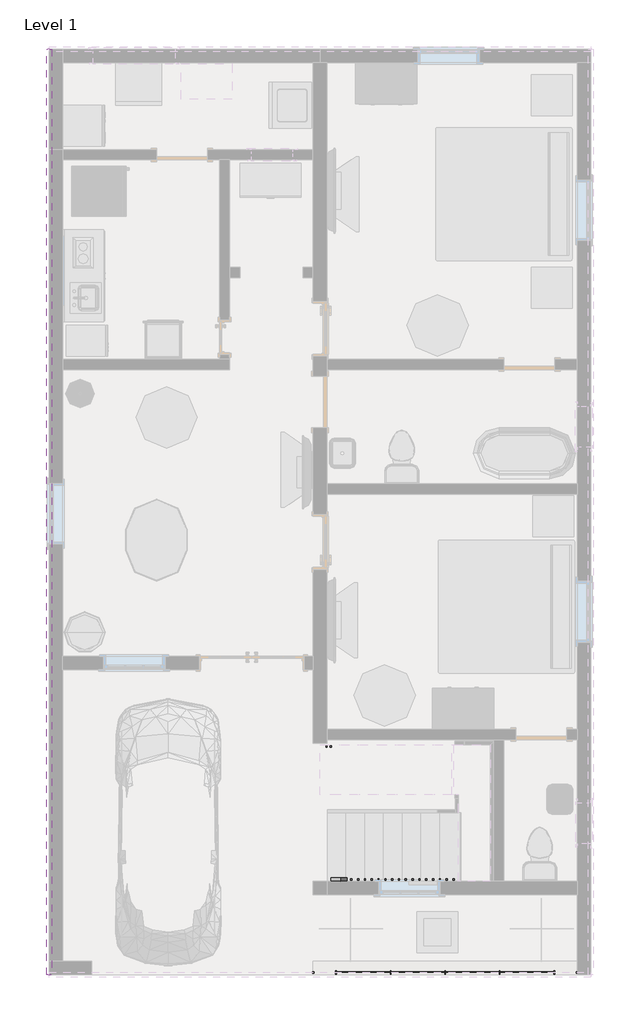
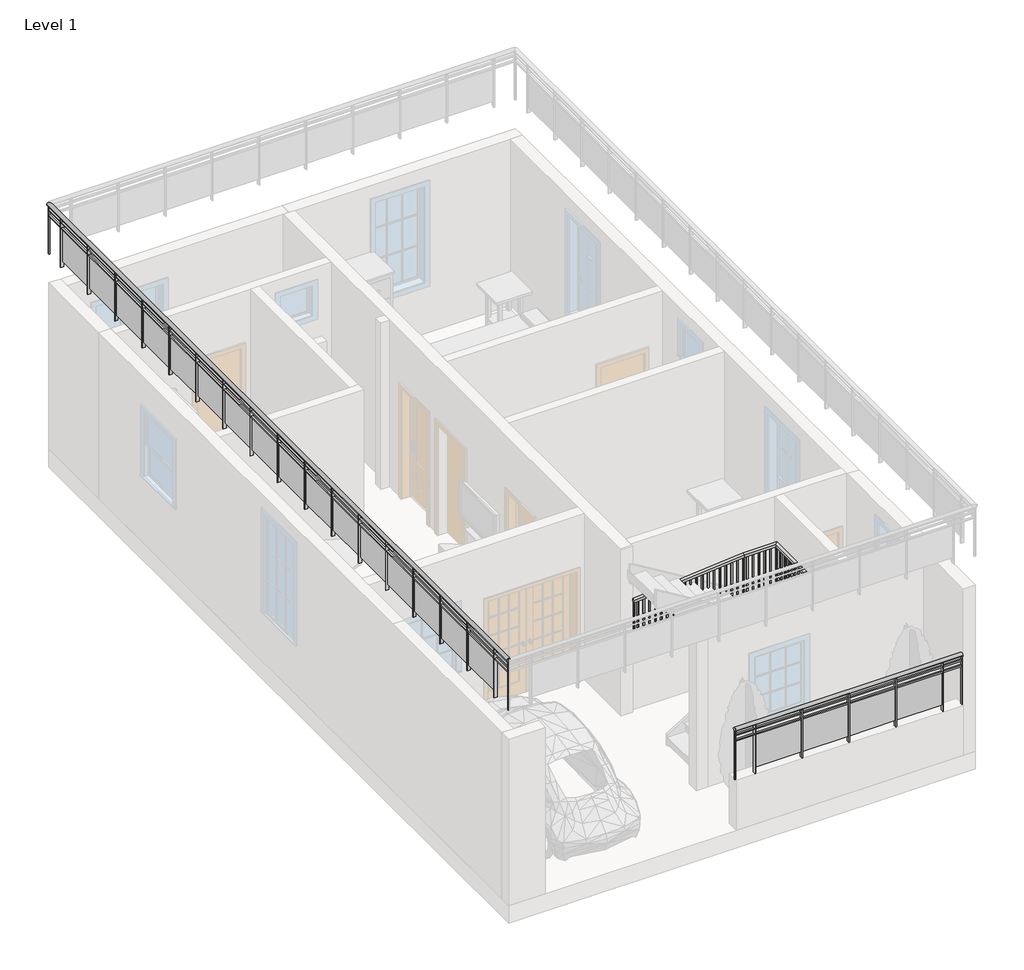
# One storey, part 2 of 3: 3 railings.
"""IFC4 building model written with IfcOpenShell, lengths in millimetres."""

from ifc_helpers import new_model, si_unit, point, frame, origin, place, context, project, spatial, polyline, ellipse_curve, trimmed, outline, extrude, faceted_brep, element, save
from ifc_brep_helpers import plane_surface, extruded_surface, advanced_brep

model = new_model("IFC4")

# Units and contexts
model_context = context("Model", 3, world=origin())
ifc_project = project(units=[si_unit("LENGTHUNIT", "METRE", prefix="MILLI")], contexts=[model_context])

# Site, building, storey
site = spatial("IfcSite", under=ifc_project)
building = spatial("IfcBuilding", under=site)
storey = spatial("IfcBuildingStorey", under=building, Name="Level 1", Elevation=0.0)

# Railings
placement = place(None, origin())
element("IfcRailing", 1, ObjectType="Glass Panel - Bottom Fill", at=placement, inside=storey, context=model_context, shape_type="SolidModel", body=[
    advanced_brep(
    [(-12539.0873398, 11712.5033005, 4495.8), (-12615.2873398, 11712.5033005, 4495.8), (-12539.0873398, -2079.6966995, 4495.8), (-12615.2873398, -2079.6966995, 4495.8)],
    [
        (0, 1, ellipse_curve(frame((-12577.1873398, 11712.5033005, 4495.8), z_axis=(0.0, 1.0, 0.0), x_axis=(-1.0, 0.0, 0.0)), 38.1, 28.575)),
        (1, 0, ellipse_curve(frame((-12577.1873398, 11712.5033005, 4495.8), z_axis=(0.0, 1.0, 0.0), x_axis=(-1.0, 0.0, 0.0)), 38.1, 28.575)),
        (2, 3, ellipse_curve(frame((-12577.1873398, -2079.6966995, 4495.8), z_axis=(0.0, -1.0, 0.0), x_axis=(-1.0, 0.0, 0.0)), 38.1, 28.575)),
        (3, 2, ellipse_curve(frame((-12577.1873398, -2079.6966995, 4495.8), z_axis=(0.0, -1.0, 0.0), x_axis=(-1.0, 0.0, 0.0)), 38.1, 28.575)),
        (0, 2),
        (3, 1),
    ],
    [
        plane_surface(frame((-12577.1873398, 11712.5033005, 4495.8), z_axis=(0.0, 1.0, 0.0), x_axis=(0.0, 0.0, -1.0))),
        plane_surface(frame((-12577.1873398, -2079.6966995, 4495.8), z_axis=(0.0, -1.0, 0.0), x_axis=(0.0, 0.0, -1.0))),
        extruded_surface(trimmed(ellipse_curve(frame((-12577.1873398, -2079.6966995, 4495.8), z_axis=(0.0, 1.0, 0.0), x_axis=(-1.0, 0.0, 0.0)), 38.1, 28.575), [point((-12539.0873398, -2079.6966995, 4495.8))], [point((-12615.2873398, -2079.6966995, 4495.8))], True, "CARTESIAN"), (0.0, 13792.2, 0.0), 13792.2),
        extruded_surface(trimmed(ellipse_curve(frame((-12577.1873398, -2079.6966995, 4495.8), z_axis=(0.0, 1.0, 0.0), x_axis=(-1.0, 0.0, 0.0)), 38.1, 28.575), [point((-12615.2873398, -2079.6966995, 4495.8))], [point((-12539.0873398, -2079.6966995, 4495.8))], True, "CARTESIAN"), (0.0, 13792.2, 0.0), 13792.2),
    ],
    [
        (0, [[1, 2]]),
        (1, [[3, 4]]),
        (2, [[-1, 5, -4, 6]]),
        (3, [[-2, -6, -3, -5]]),
    ],
),
    extrude(outline(polyline([(-12589.8873398, 11712.5033005), (-12564.4873398, 11712.5033005), (-12564.4873398, -2079.6966995), (-12589.8873398, -2079.6966995), (-12589.8873398, 11712.5033005)])), frame((0.0, 0.0, 4381.5), z_axis=(0.0, 0.0, 1.0), x_axis=(1.0, 0.0, 0.0)), (0.0, 0.0, 1.0), 25.4),
    extrude(outline(polyline([(-12589.8873398, 11712.5033005), (-12564.4873398, 11712.5033005), (-12564.4873398, -2079.6966995), (-12589.8873398, -2079.6966995), (-12589.8873398, 11712.5033005)])), frame((0.0, 0.0, 4279.9), z_axis=(0.0, 0.0, 1.0), x_axis=(1.0, 0.0, 0.0)), (0.0, 0.0, 1.0), 25.4),
    extrude(outline(polyline([(-12602.5873398, -1679.6466995), (-12551.7873398, -1679.6466995), (-12551.7873398, -1692.3466995), (-12602.5873398, -1692.3466995), (-12602.5873398, -1679.6466995)])), frame((0.0, 0.0, 3581.4), z_axis=(0.0, 0.0, 1.0), x_axis=(1.0, 0.0, 0.0)), (0.0, 0.0, 1.0), 885.6788223),
    extrude(outline(polyline([(-12570.6521828, -873.1966995), (-12570.6521828, -1685.9966995), (-12577.0021828, -1685.9966995), (-12577.0021828, -873.1966995), (-12570.6521828, -873.1966995)])), frame((0.0, 0.0, 3683.0), z_axis=(0.0, 0.0, 1.0), x_axis=(1.0, 0.0, 0.0)), (0.0, 0.0, 1.0), 596.9),
    extrude(outline(polyline([(-12602.5873398, -866.8466995), (-12551.7873398, -866.8466995), (-12551.7873398, -879.5466995), (-12602.5873398, -879.5466995), (-12602.5873398, -866.8466995)])), frame((0.0, 0.0, 3581.4), z_axis=(0.0, 0.0, 1.0), x_axis=(1.0, 0.0, 0.0)), (0.0, 0.0, 1.0), 885.6788223),
    extrude(outline(polyline([(-12570.6521828, -60.3966995), (-12570.6521828, -873.1966995), (-12577.0021828, -873.1966995), (-12577.0021828, -60.3966995), (-12570.6521828, -60.3966995)])), frame((0.0, 0.0, 3683.0), z_axis=(0.0, 0.0, 1.0), x_axis=(1.0, 0.0, 0.0)), (0.0, 0.0, 1.0), 596.9),
    extrude(outline(polyline([(-12602.5873398, -54.0466995), (-12551.7873398, -54.0466995), (-12551.7873398, -66.7466995), (-12602.5873398, -66.7466995), (-12602.5873398, -54.0466995)])), frame((0.0, 0.0, 3581.4), z_axis=(0.0, 0.0, 1.0), x_axis=(1.0, 0.0, 0.0)), (0.0, 0.0, 1.0), 885.6788223),
    extrude(outline(polyline([(-12570.6521828, 752.4033005), (-12570.6521828, -60.3966995), (-12577.0021828, -60.3966995), (-12577.0021828, 752.4033005), (-12570.6521828, 752.4033005)])), frame((0.0, 0.0, 3683.0), z_axis=(0.0, 0.0, 1.0), x_axis=(1.0, 0.0, 0.0)), (0.0, 0.0, 1.0), 596.9),
    extrude(outline(polyline([(-12602.5873398, 758.7533005), (-12551.7873398, 758.7533005), (-12551.7873398, 746.0533005), (-12602.5873398, 746.0533005), (-12602.5873398, 758.7533005)])), frame((0.0, 0.0, 3581.4), z_axis=(0.0, 0.0, 1.0), x_axis=(1.0, 0.0, 0.0)), (0.0, 0.0, 1.0), 885.6788223),
    extrude(outline(polyline([(-12570.6521828, 1565.2033005), (-12570.6521828, 752.4033005), (-12577.0021828, 752.4033005), (-12577.0021828, 1565.2033005), (-12570.6521828, 1565.2033005)])), frame((0.0, 0.0, 3683.0), z_axis=(0.0, 0.0, 1.0), x_axis=(1.0, 0.0, 0.0)), (0.0, 0.0, 1.0), 596.9),
    extrude(outline(polyline([(-12602.5873398, 1571.5533005), (-12551.7873398, 1571.5533005), (-12551.7873398, 1558.8533005), (-12602.5873398, 1558.8533005), (-12602.5873398, 1571.5533005)])), frame((0.0, 0.0, 3581.4), z_axis=(0.0, 0.0, 1.0), x_axis=(1.0, 0.0, 0.0)), (0.0, 0.0, 1.0), 885.6788223),
    extrude(outline(polyline([(-12570.6521828, 2378.0033005), (-12570.6521828, 1565.2033005), (-12577.0021828, 1565.2033005), (-12577.0021828, 2378.0033005), (-12570.6521828, 2378.0033005)])), frame((0.0, 0.0, 3683.0), z_axis=(0.0, 0.0, 1.0), x_axis=(1.0, 0.0, 0.0)), (0.0, 0.0, 1.0), 596.9),
    extrude(outline(polyline([(-12602.5873398, 2384.3533005), (-12551.7873398, 2384.3533005), (-12551.7873398, 2371.6533005), (-12602.5873398, 2371.6533005), (-12602.5873398, 2384.3533005)])), frame((0.0, 0.0, 3581.4), z_axis=(0.0, 0.0, 1.0), x_axis=(1.0, 0.0, 0.0)), (0.0, 0.0, 1.0), 885.6788223),
    extrude(outline(polyline([(-12570.6521828, 3190.8033005), (-12570.6521828, 2378.0033005), (-12577.0021828, 2378.0033005), (-12577.0021828, 3190.8033005), (-12570.6521828, 3190.8033005)])), frame((0.0, 0.0, 3683.0), z_axis=(0.0, 0.0, 1.0), x_axis=(1.0, 0.0, 0.0)), (0.0, 0.0, 1.0), 596.9),
    extrude(outline(polyline([(-12602.5873398, 3197.1533005), (-12551.7873398, 3197.1533005), (-12551.7873398, 3184.4533005), (-12602.5873398, 3184.4533005), (-12602.5873398, 3197.1533005)])), frame((0.0, 0.0, 3581.4), z_axis=(0.0, 0.0, 1.0), x_axis=(1.0, 0.0, 0.0)), (0.0, 0.0, 1.0), 885.6788223),
    extrude(outline(polyline([(-12570.6521828, 4003.6033005), (-12570.6521828, 3190.8033005), (-12577.0021828, 3190.8033005), (-12577.0021828, 4003.6033005), (-12570.6521828, 4003.6033005)])), frame((0.0, 0.0, 3683.0), z_axis=(0.0, 0.0, 1.0), x_axis=(1.0, 0.0, 0.0)), (0.0, 0.0, 1.0), 596.9),
    extrude(outline(polyline([(-12602.5873398, 4009.9533005), (-12551.7873398, 4009.9533005), (-12551.7873398, 3997.2533005), (-12602.5873398, 3997.2533005), (-12602.5873398, 4009.9533005)])), frame((0.0, 0.0, 3581.4), z_axis=(0.0, 0.0, 1.0), x_axis=(1.0, 0.0, 0.0)), (0.0, 0.0, 1.0), 885.6788223),
    extrude(outline(polyline([(-12570.6521828, 4816.4033005), (-12570.6521828, 4003.6033005), (-12577.0021828, 4003.6033005), (-12577.0021828, 4816.4033005), (-12570.6521828, 4816.4033005)])), frame((0.0, 0.0, 3683.0), z_axis=(0.0, 0.0, 1.0), x_axis=(1.0, 0.0, 0.0)), (0.0, 0.0, 1.0), 596.9),
    extrude(outline(polyline([(-12602.5873398, 4822.7533005), (-12551.7873398, 4822.7533005), (-12551.7873398, 4810.0533005), (-12602.5873398, 4810.0533005), (-12602.5873398, 4822.7533005)])), frame((0.0, 0.0, 3581.4), z_axis=(0.0, 0.0, 1.0), x_axis=(1.0, 0.0, 0.0)), (0.0, 0.0, 1.0), 885.6788223),
    extrude(outline(polyline([(-12570.6521828, 5629.2033005), (-12570.6521828, 4816.4033005), (-12577.0021828, 4816.4033005), (-12577.0021828, 5629.2033005), (-12570.6521828, 5629.2033005)])), frame((0.0, 0.0, 3683.0), z_axis=(0.0, 0.0, 1.0), x_axis=(1.0, 0.0, 0.0)), (0.0, 0.0, 1.0), 596.9),
    extrude(outline(polyline([(-12602.5873398, 5635.5533005), (-12551.7873398, 5635.5533005), (-12551.7873398, 5622.8533005), (-12602.5873398, 5622.8533005), (-12602.5873398, 5635.5533005)])), frame((0.0, 0.0, 3581.4), z_axis=(0.0, 0.0, 1.0), x_axis=(1.0, 0.0, 0.0)), (0.0, 0.0, 1.0), 885.6788223),
    extrude(outline(polyline([(-12570.6521828, 6442.0033005), (-12570.6521828, 5629.2033005), (-12577.0021828, 5629.2033005), (-12577.0021828, 6442.0033005), (-12570.6521828, 6442.0033005)])), frame((0.0, 0.0, 3683.0), z_axis=(0.0, 0.0, 1.0), x_axis=(1.0, 0.0, 0.0)), (0.0, 0.0, 1.0), 596.9),
    extrude(outline(polyline([(-12602.5873398, 6448.3533005), (-12551.7873398, 6448.3533005), (-12551.7873398, 6435.6533005), (-12602.5873398, 6435.6533005), (-12602.5873398, 6448.3533005)])), frame((0.0, 0.0, 3581.4), z_axis=(0.0, 0.0, 1.0), x_axis=(1.0, 0.0, 0.0)), (0.0, 0.0, 1.0), 885.6788223),
    extrude(outline(polyline([(-12570.6521828, 7254.8033005), (-12570.6521828, 6442.0033005), (-12577.0021828, 6442.0033005), (-12577.0021828, 7254.8033005), (-12570.6521828, 7254.8033005)])), frame((0.0, 0.0, 3683.0), z_axis=(0.0, 0.0, 1.0), x_axis=(1.0, 0.0, 0.0)), (0.0, 0.0, 1.0), 596.9),
    extrude(outline(polyline([(-12602.5873398, 7261.1533005), (-12551.7873398, 7261.1533005), (-12551.7873398, 7248.4533005), (-12602.5873398, 7248.4533005), (-12602.5873398, 7261.1533005)])), frame((0.0, 0.0, 3581.4), z_axis=(0.0, 0.0, 1.0), x_axis=(1.0, 0.0, 0.0)), (0.0, 0.0, 1.0), 885.6788223),
    extrude(outline(polyline([(-12570.6521828, 8067.6033005), (-12570.6521828, 7254.8033005), (-12577.0021828, 7254.8033005), (-12577.0021828, 8067.6033005), (-12570.6521828, 8067.6033005)])), frame((0.0, 0.0, 3683.0), z_axis=(0.0, 0.0, 1.0), x_axis=(1.0, 0.0, 0.0)), (0.0, 0.0, 1.0), 596.9),
    extrude(outline(polyline([(-12602.5873398, 8073.9533005), (-12551.7873398, 8073.9533005), (-12551.7873398, 8061.2533005), (-12602.5873398, 8061.2533005), (-12602.5873398, 8073.9533005)])), frame((0.0, 0.0, 3581.4), z_axis=(0.0, 0.0, 1.0), x_axis=(1.0, 0.0, 0.0)), (0.0, 0.0, 1.0), 885.6788223),
    extrude(outline(polyline([(-12570.6521828, 8880.4033005), (-12570.6521828, 8067.6033005), (-12577.0021828, 8067.6033005), (-12577.0021828, 8880.4033005), (-12570.6521828, 8880.4033005)])), frame((0.0, 0.0, 3683.0), z_axis=(0.0, 0.0, 1.0), x_axis=(1.0, 0.0, 0.0)), (0.0, 0.0, 1.0), 596.9),
    extrude(outline(polyline([(-12602.5873398, 8886.7533005), (-12551.7873398, 8886.7533005), (-12551.7873398, 8874.0533005), (-12602.5873398, 8874.0533005), (-12602.5873398, 8886.7533005)])), frame((0.0, 0.0, 3581.4), z_axis=(0.0, 0.0, 1.0), x_axis=(1.0, 0.0, 0.0)), (0.0, 0.0, 1.0), 885.6788223),
    extrude(outline(polyline([(-12570.6521828, 9693.2033005), (-12570.6521828, 8880.4033005), (-12577.0021828, 8880.4033005), (-12577.0021828, 9693.2033005), (-12570.6521828, 9693.2033005)])), frame((0.0, 0.0, 3683.0), z_axis=(0.0, 0.0, 1.0), x_axis=(1.0, 0.0, 0.0)), (0.0, 0.0, 1.0), 596.9),
    extrude(outline(polyline([(-12602.5873398, 9699.5533005), (-12551.7873398, 9699.5533005), (-12551.7873398, 9686.8533005), (-12602.5873398, 9686.8533005), (-12602.5873398, 9699.5533005)])), frame((0.0, 0.0, 3581.4), z_axis=(0.0, 0.0, 1.0), x_axis=(1.0, 0.0, 0.0)), (0.0, 0.0, 1.0), 885.6788223),
    extrude(outline(polyline([(-12570.6521828, 10506.0033005), (-12570.6521828, 9693.2033005), (-12577.0021828, 9693.2033005), (-12577.0021828, 10506.0033005), (-12570.6521828, 10506.0033005)])), frame((0.0, 0.0, 3683.0), z_axis=(0.0, 0.0, 1.0), x_axis=(1.0, 0.0, 0.0)), (0.0, 0.0, 1.0), 596.9),
    extrude(outline(polyline([(-12602.5873398, 10512.3533005), (-12551.7873398, 10512.3533005), (-12551.7873398, 10499.6533005), (-12602.5873398, 10499.6533005), (-12602.5873398, 10512.3533005)])), frame((0.0, 0.0, 3581.4), z_axis=(0.0, 0.0, 1.0), x_axis=(1.0, 0.0, 0.0)), (0.0, 0.0, 1.0), 885.6788223),
    extrude(outline(polyline([(-12570.6521828, 11318.8033005), (-12570.6521828, 10506.0033005), (-12577.0021828, 10506.0033005), (-12577.0021828, 11318.8033005), (-12570.6521828, 11318.8033005)])), frame((0.0, 0.0, 3683.0), z_axis=(0.0, 0.0, 1.0), x_axis=(1.0, 0.0, 0.0)), (0.0, 0.0, 1.0), 596.9),
    extrude(outline(polyline([(-12602.5873398, 11325.1533005), (-12551.7873398, 11325.1533005), (-12551.7873398, 11312.4533005), (-12602.5873398, 11312.4533005), (-12602.5873398, 11325.1533005)])), frame((0.0, 0.0, 3581.4), z_axis=(0.0, 0.0, 1.0), x_axis=(1.0, 0.0, 0.0)), (0.0, 0.0, 1.0), 885.6788223),
    extrude(outline(polyline([(-12586.7123398, -2066.9966995), (-12567.6623398, -2066.9966995), (-12567.6623398, -2086.0466995), (-12586.7123398, -2086.0466995), (-12586.7123398, -2066.9966995)])), frame((0.0, 0.0, 3581.4), z_axis=(0.0, 0.0, 1.0), x_axis=(1.0, 0.0, 0.0)), (0.0, 0.0, 1.0), 885.6788223),
    extrude(outline(polyline([(-12586.7123398, 11718.8533005), (-12567.6623398, 11718.8533005), (-12567.6623398, 11699.8033005), (-12586.7123398, 11699.8033005), (-12586.7123398, 11718.8533005)])), frame((0.0, 0.0, 3581.4), z_axis=(0.0, 0.0, 1.0), x_axis=(1.0, 0.0, 0.0)), (0.0, 0.0, 1.0), 885.6788223),
])
element("IfcRailing", 2, ObjectType="Glass Panel - Bottom Fill", at=placement, inside=storey, context=model_context, shape_type="SolidModel", body=[
    advanced_brep(
    [(-8640.1873398, -2003.4966995, 1828.8), (-8640.1873398, -2079.6966995, 1828.8), (-4703.1873398, -2003.4966995, 1828.8), (-4703.1873398, -2079.6966995, 1828.8)],
    [
        (0, 1, ellipse_curve(frame((-8640.1873398, -2041.5966995, 1828.8), z_axis=(-1.0, 0.0, 0.0), x_axis=(0.0, -1.0, 0.0)), 38.1, 28.575)),
        (1, 0, ellipse_curve(frame((-8640.1873398, -2041.5966995, 1828.8), z_axis=(-1.0, 0.0, 0.0), x_axis=(0.0, -1.0, 0.0)), 38.1, 28.575)),
        (2, 3, ellipse_curve(frame((-4703.1873398, -2041.5966995, 1828.8), z_axis=(1.0, 0.0, 0.0), x_axis=(0.0, -1.0, 0.0)), 38.1, 28.575)),
        (3, 2, ellipse_curve(frame((-4703.1873398, -2041.5966995, 1828.8), z_axis=(1.0, 0.0, 0.0), x_axis=(0.0, -1.0, 0.0)), 38.1, 28.575)),
        (0, 2),
        (3, 1),
    ],
    [
        plane_surface(frame((-8640.1873398, -2041.5966995, 1828.8), z_axis=(-1.0, 0.0, 0.0), x_axis=(0.0, 1.0, 0.0))),
        plane_surface(frame((-4703.1873398, -2041.5966995, 1828.8), z_axis=(1.0, 0.0, 0.0), x_axis=(0.0, 1.0, 0.0))),
        extruded_surface(trimmed(ellipse_curve(frame((-4703.1873398, -2041.5966995, 1828.8), z_axis=(-1.0, 0.0, 0.0), x_axis=(0.0, -1.0, 0.0)), 38.1, 28.575), [point((-4703.1873398, -2003.4966995, 1828.8))], [point((-4703.1873398, -2079.6966995, 1828.8))], True, "CARTESIAN"), (-3937.000000000001, 0.0, 0.0), 3937.000000000001),
        extruded_surface(trimmed(ellipse_curve(frame((-4703.1873398, -2041.5966995, 1828.8), z_axis=(-1.0, 0.0, 0.0), x_axis=(0.0, -1.0, 0.0)), 38.1, 28.575), [point((-4703.1873398, -2079.6966995, 1828.8))], [point((-4703.1873398, -2003.4966995, 1828.8))], True, "CARTESIAN"), (-3937.000000000001, 0.0, 0.0), 3937.000000000001),
    ],
    [
        (0, [[1, 2]]),
        (1, [[3, 4]]),
        (2, [[-1, 5, -4, 6]]),
        (3, [[-2, -6, -3, -5]]),
    ],
),
    extrude(outline(polyline([(-8640.1873398, -2054.2966995), (-8640.1873398, -2028.8966995), (-4703.1873398, -2028.8966995), (-4703.1873398, -2054.2966995), (-8640.1873398, -2054.2966995)])), frame((0.0, 0.0, 1714.5), z_axis=(0.0, 0.0, 1.0), x_axis=(1.0, 0.0, 0.0)), (0.0, 0.0, 1.0), 25.4),
    extrude(outline(polyline([(-8640.1873398, -2054.2966995), (-8640.1873398, -2028.8966995), (-4703.1873398, -2028.8966995), (-4703.1873398, -2054.2966995), (-8640.1873398, -2054.2966995)])), frame((0.0, 0.0, 1612.9), z_axis=(0.0, 0.0, 1.0), x_axis=(1.0, 0.0, 0.0)), (0.0, 0.0, 1.0), 25.4),
    extrude(outline(polyline([(-5052.4373398, -2066.9966995), (-5052.4373398, -2016.1966995), (-5039.7373398, -2016.1966995), (-5039.7373398, -2066.9966995), (-5052.4373398, -2066.9966995)])), frame((0.0, 0.0, 914.4), z_axis=(0.0, 0.0, 1.0), x_axis=(1.0, 0.0, 0.0)), (0.0, 0.0, 1.0), 885.6788223),
    extrude(outline(polyline([(-5858.8873398, -2035.0615425), (-5046.0873398, -2035.0615425), (-5046.0873398, -2041.4115425), (-5858.8873398, -2041.4115425), (-5858.8873398, -2035.0615425)])), frame((0.0, 0.0, 1016.0), z_axis=(0.0, 0.0, 1.0), x_axis=(1.0, 0.0, 0.0)), (0.0, 0.0, 1.0), 596.9),
    extrude(outline(polyline([(-5865.2373398, -2066.9966995), (-5865.2373398, -2016.1966995), (-5852.5373398, -2016.1966995), (-5852.5373398, -2066.9966995), (-5865.2373398, -2066.9966995)])), frame((0.0, 0.0, 914.4), z_axis=(0.0, 0.0, 1.0), x_axis=(1.0, 0.0, 0.0)), (0.0, 0.0, 1.0), 885.6788223),
    extrude(outline(polyline([(-6671.6873398, -2035.0615425), (-5858.8873398, -2035.0615425), (-5858.8873398, -2041.4115425), (-6671.6873398, -2041.4115425), (-6671.6873398, -2035.0615425)])), frame((0.0, 0.0, 1016.0), z_axis=(0.0, 0.0, 1.0), x_axis=(1.0, 0.0, 0.0)), (0.0, 0.0, 1.0), 596.9),
    extrude(outline(polyline([(-6678.0373398, -2066.9966995), (-6678.0373398, -2016.1966995), (-6665.3373398, -2016.1966995), (-6665.3373398, -2066.9966995), (-6678.0373398, -2066.9966995)])), frame((0.0, 0.0, 914.4), z_axis=(0.0, 0.0, 1.0), x_axis=(1.0, 0.0, 0.0)), (0.0, 0.0, 1.0), 885.6788223),
    extrude(outline(polyline([(-7484.4873398, -2035.0615425), (-6671.6873398, -2035.0615425), (-6671.6873398, -2041.4115425), (-7484.4873398, -2041.4115425), (-7484.4873398, -2035.0615425)])), frame((0.0, 0.0, 1016.0), z_axis=(0.0, 0.0, 1.0), x_axis=(1.0, 0.0, 0.0)), (0.0, 0.0, 1.0), 596.9),
    extrude(outline(polyline([(-7490.8373398, -2066.9966995), (-7490.8373398, -2016.1966995), (-7478.1373398, -2016.1966995), (-7478.1373398, -2066.9966995), (-7490.8373398, -2066.9966995)])), frame((0.0, 0.0, 914.4), z_axis=(0.0, 0.0, 1.0), x_axis=(1.0, 0.0, 0.0)), (0.0, 0.0, 1.0), 885.6788223),
    extrude(outline(polyline([(-8297.2873398, -2035.0615425), (-7484.4873398, -2035.0615425), (-7484.4873398, -2041.4115425), (-8297.2873398, -2041.4115425), (-8297.2873398, -2035.0615425)])), frame((0.0, 0.0, 1016.0), z_axis=(0.0, 0.0, 1.0), x_axis=(1.0, 0.0, 0.0)), (0.0, 0.0, 1.0), 596.9),
    extrude(outline(polyline([(-8303.6373398, -2066.9966995), (-8303.6373398, -2016.1966995), (-8290.9373398, -2016.1966995), (-8290.9373398, -2066.9966995), (-8303.6373398, -2066.9966995)])), frame((0.0, 0.0, 914.4), z_axis=(0.0, 0.0, 1.0), x_axis=(1.0, 0.0, 0.0)), (0.0, 0.0, 1.0), 885.6788223),
    extrude(outline(polyline([(-4715.8873398, -2051.1216995), (-4715.8873398, -2032.0716995), (-4696.8373398, -2032.0716995), (-4696.8373398, -2051.1216995), (-4715.8873398, -2051.1216995)])), frame((0.0, 0.0, 914.4), z_axis=(0.0, 0.0, 1.0), x_axis=(1.0, 0.0, 0.0)), (0.0, 0.0, 1.0), 885.6788223),
    extrude(outline(polyline([(-8646.5373398, -2051.1216995), (-8646.5373398, -2032.0716995), (-8627.4873398, -2032.0716995), (-8627.4873398, -2051.1216995), (-8646.5373398, -2051.1216995)])), frame((0.0, 0.0, 914.4), z_axis=(0.0, 0.0, 1.0), x_axis=(1.0, 0.0, 0.0)), (0.0, 0.0, 1.0), 885.6788223),
])
element("IfcRailing", 3, ObjectType="Handrail - Rectangular", at=placement, inside=storey, context=model_context, shape_type="SolidModel", body=[
    faceted_brep([(-8451.9655018, 1298.0576368, 2104.1316017), (-8451.9655018, 1348.8576368, 2104.1316017), (-8451.9655018, 1348.8576368, 2053.141556), (-8451.9655018, 1298.0576368, 2053.141556), (-6544.7704735, 1298.0576368, 2218.2666667), (-6546.9655018, 1298.0576368, 2269.0666667), (-6544.7704735, 1348.8576368, 2218.2666667), (-6546.9655018, 1348.8576368, 2269.0666667), (-5999.5047162, -631.8966995, 2218.2666667), (-5999.5047162, -631.8966995, 2269.0666667), (-5999.5047162, 1298.0576368, 2269.0666667), (-5999.5047162, 1298.0576368, 2218.2666667), (-5948.7047162, -682.6966995, 2218.2666667), (-5948.7047162, 1348.8576368, 2218.2666667), (-5948.7047162, -682.6966995, 2269.0666667), (-5948.7047162, 1348.8576368, 2269.0666667), (-8375.7655018, -631.8966995, 1114.5212121), (-8375.7655018, -631.8966995, 1055.1197519), (-8375.7655018, -682.6966995, 1055.1197519), (-8375.7655018, -682.6966995, 1114.5212121), (-6470.7655018, -631.8966995, 2269.0666667), (-6456.5730924, -631.8966995, 2218.2666667), (-6456.5730924, -682.6966995, 2218.2666667), (-6470.7655018, -682.6966995, 2269.0666667)], [[[0, 1, 2, 3]], [[4, 5, 0, 3]], [[6, 4, 3, 2]], [[7, 6, 2, 1]], [[5, 7, 1, 0]], [[8, 9, 10, 11]], [[12, 8, 11, 13]], [[14, 12, 13, 15]], [[9, 14, 15, 10]], [[11, 10, 5, 4]], [[13, 11, 4, 6]], [[15, 13, 6, 7]], [[10, 15, 7, 5]], [[16, 17, 18, 19]], [[17, 16, 20, 21]], [[18, 17, 21, 22]], [[19, 18, 22, 23]], [[16, 19, 23, 20]], [[21, 20, 9, 8]], [[22, 21, 8, 12]], [[23, 22, 12, 14]], [[20, 23, 14, 9]]]),
    extrude(outline(polyline([(2060.5636339, -8366.2405018), (2058.9142833, -8385.2905018), (1196.3290043, -8385.2905018), (1196.3290043, -8366.2405018), (2060.5636339, -8366.2405018)])), frame((0.0, 1313.9326368, 0.0), z_axis=(0.0, 1.0, 0.0), x_axis=(0.0, 0.0, 1.0)), (0.0, 0.0, 1.0), 19.05),
    extrude(outline(polyline([(2069.3601707, -8264.6405018), (2067.7108201, -8283.6905018), (1205.1255411, -8283.6905018), (1205.1255411, -8264.6405018), (2069.3601707, -8264.6405018)])), frame((0.0, 1313.9326368, 0.0), z_axis=(0.0, 1.0, 0.0), x_axis=(0.0, 0.0, 1.0)), (0.0, 0.0, 1.0), 19.05),
    extrude(outline(polyline([(2078.1567075, -8163.0405018), (2076.5073569, -8182.0905018), (1213.9220779, -8182.0905018), (1213.9220779, -8163.0405018), (2078.1567075, -8163.0405018)])), frame((0.0, 1313.9326368, 0.0), z_axis=(0.0, 1.0, 0.0), x_axis=(0.0, 0.0, 1.0)), (0.0, 0.0, 1.0), 19.05),
    extrude(outline(polyline([(2086.9532443, -8061.4405018), (2085.3038937, -8080.4905018), (1222.7186147, -8080.4905018), (1222.7186147, -8061.4405018), (2086.9532443, -8061.4405018)])), frame((0.0, 1313.9326368, 0.0), z_axis=(0.0, 1.0, 0.0), x_axis=(0.0, 0.0, 1.0)), (0.0, 0.0, 1.0), 19.05),
    extrude(outline(polyline([(2095.7497811, -7959.8405018), (2094.1004304, -7978.8905018), (1231.5151515, -7978.8905018), (1231.5151515, -7959.8405018), (2095.7497811, -7959.8405018)])), frame((0.0, 1313.9326368, 0.0), z_axis=(0.0, 1.0, 0.0), x_axis=(0.0, 0.0, 1.0)), (0.0, 0.0, 1.0), 19.05),
    extrude(outline(polyline([(2104.5463179, -7858.2405018), (2102.8969672, -7877.2905018), (1240.3116883, -7877.2905018), (1240.3116883, -7858.2405018), (2104.5463179, -7858.2405018)])), frame((0.0, 1313.9326368, 0.0), z_axis=(0.0, 1.0, 0.0), x_axis=(0.0, 0.0, 1.0)), (0.0, 0.0, 1.0), 19.05),
    extrude(outline(polyline([(2113.3428547, -7756.6405018), (2111.693504, -7775.6905018), (1249.1082251, -7775.6905018), (1249.1082251, -7756.6405018), (2113.3428547, -7756.6405018)])), frame((0.0, 1313.9326368, 0.0), z_axis=(0.0, 1.0, 0.0), x_axis=(0.0, 0.0, 1.0)), (0.0, 0.0, 1.0), 19.05),
    extrude(outline(polyline([(2122.1393915, -7655.0405018), (2120.4900408, -7674.0905018), (2032.0, -7674.0905018), (2032.0, -7655.0405018), (2122.1393915, -7655.0405018)])), frame((0.0, 1313.9326368, 0.0), z_axis=(0.0, 1.0, 0.0), x_axis=(0.0, 0.0, 1.0)), (0.0, 0.0, 1.0), 19.05),
    extrude(outline(polyline([(2130.9359283, -7553.4405018), (2129.2865776, -7572.4905018), (2032.0, -7572.4905018), (2032.0, -7553.4405018), (2130.9359283, -7553.4405018)])), frame((0.0, 1313.9326368, 0.0), z_axis=(0.0, 1.0, 0.0), x_axis=(0.0, 0.0, 1.0)), (0.0, 0.0, 1.0), 19.05),
    extrude(outline(polyline([(2139.7324651, -7451.8405018), (2138.0831144, -7470.8905018), (2032.0, -7470.8905018), (2032.0, -7451.8405018), (2139.7324651, -7451.8405018)])), frame((0.0, 1313.9326368, 0.0), z_axis=(0.0, 1.0, 0.0), x_axis=(0.0, 0.0, 1.0)), (0.0, 0.0, 1.0), 19.05),
    extrude(outline(polyline([(2148.5290019, -7350.2405018), (2146.8796512, -7369.2905018), (1862.6666667, -7369.2905018), (1862.6666667, -7350.2405018), (2148.5290019, -7350.2405018)])), frame((0.0, 1313.9326368, 0.0), z_axis=(0.0, 1.0, 0.0), x_axis=(0.0, 0.0, 1.0)), (0.0, 0.0, 1.0), 19.05),
    extrude(outline(polyline([(2157.3255387, -7248.6405018), (2155.676188, -7267.6905018), (1862.6666667, -7267.6905018), (1862.6666667, -7248.6405018), (2157.3255387, -7248.6405018)])), frame((0.0, 1313.9326368, 0.0), z_axis=(0.0, 1.0, 0.0), x_axis=(0.0, 0.0, 1.0)), (0.0, 0.0, 1.0), 19.05),
    extrude(outline(polyline([(2166.1220755, -7147.0405018), (2164.4727248, -7166.0905018), (1862.6666667, -7166.0905018), (1862.6666667, -7147.0405018), (2166.1220755, -7147.0405018)])), frame((0.0, 1313.9326368, 0.0), z_axis=(0.0, 1.0, 0.0), x_axis=(0.0, 0.0, 1.0)), (0.0, 0.0, 1.0), 19.05),
    extrude(outline(polyline([(2174.9186123, -7045.4405018), (2173.2692616, -7064.4905018), (1693.3333333, -7064.4905018), (1693.3333333, -7045.4405018), (2174.9186123, -7045.4405018)])), frame((0.0, 1313.9326368, 0.0), z_axis=(0.0, 1.0, 0.0), x_axis=(0.0, 0.0, 1.0)), (0.0, 0.0, 1.0), 19.05),
    extrude(outline(polyline([(2183.7151491, -6943.8405018), (2182.0657984, -6962.8905018), (1693.3333333, -6962.8905018), (1693.3333333, -6943.8405018), (2183.7151491, -6943.8405018)])), frame((0.0, 1313.9326368, 0.0), z_axis=(0.0, 1.0, 0.0), x_axis=(0.0, 0.0, 1.0)), (0.0, 0.0, 1.0), 19.05),
    extrude(outline(polyline([(2192.5116859, -6842.2405018), (2190.8623352, -6861.2905018), (1693.3333333, -6861.2905018), (1693.3333333, -6842.2405018), (2192.5116859, -6842.2405018)])), frame((0.0, 1313.9326368, 0.0), z_axis=(0.0, 1.0, 0.0), x_axis=(0.0, 0.0, 1.0)), (0.0, 0.0, 1.0), 19.05),
    extrude(outline(polyline([(2201.3082227, -6740.6405018), (2199.658872, -6759.6905018), (1524.0, -6759.6905018), (1524.0, -6740.6405018), (2201.3082227, -6740.6405018)])), frame((0.0, 1313.9326368, 0.0), z_axis=(0.0, 1.0, 0.0), x_axis=(0.0, 0.0, 1.0)), (0.0, 0.0, 1.0), 19.05),
    extrude(outline(polyline([(2210.1047595, -6639.0405018), (2208.4554088, -6658.0905018), (1524.0, -6658.0905018), (1524.0, -6639.0405018), (2210.1047595, -6639.0405018)])), frame((0.0, 1313.9326368, 0.0), z_axis=(0.0, 1.0, 0.0), x_axis=(0.0, 0.0, 1.0)), (0.0, 0.0, 1.0), 19.05),
    extrude(outline(polyline([(-6472.5797162, 1332.9826368), (-6472.5797162, 1313.9326368), (-6491.6297162, 1313.9326368), (-6491.6297162, 1332.9826368), (-6472.5797162, 1332.9826368)])), frame((0.0, 0.0, 1354.6666667), z_axis=(0.0, 0.0, 1.0), x_axis=(1.0, 0.0, 0.0)), (0.0, 0.0, 1.0), 863.6),
    extrude(outline(polyline([(-6370.9797162, 1332.9826368), (-6370.9797162, 1313.9326368), (-6390.0297162, 1313.9326368), (-6390.0297162, 1332.9826368), (-6370.9797162, 1332.9826368)])), frame((0.0, 0.0, 1354.6666667), z_axis=(0.0, 0.0, 1.0), x_axis=(1.0, 0.0, 0.0)), (0.0, 0.0, 1.0), 863.6),
    extrude(outline(polyline([(-6269.3797162, 1332.9826368), (-6269.3797162, 1313.9326368), (-6288.4297162, 1313.9326368), (-6288.4297162, 1332.9826368), (-6269.3797162, 1332.9826368)])), frame((0.0, 0.0, 1354.6666667), z_axis=(0.0, 0.0, 1.0), x_axis=(1.0, 0.0, 0.0)), (0.0, 0.0, 1.0), 863.6),
    extrude(outline(polyline([(-6167.7797162, 1332.9826368), (-6167.7797162, 1313.9326368), (-6186.8297162, 1313.9326368), (-6186.8297162, 1332.9826368), (-6167.7797162, 1332.9826368)])), frame((0.0, 0.0, 1354.6666667), z_axis=(0.0, 0.0, 1.0), x_axis=(1.0, 0.0, 0.0)), (0.0, 0.0, 1.0), 863.6),
    extrude(outline(polyline([(-6066.1797162, 1332.9826368), (-6066.1797162, 1313.9326368), (-6085.2297162, 1313.9326368), (-6085.2297162, 1332.9826368), (-6066.1797162, 1332.9826368)])), frame((0.0, 0.0, 1354.6666667), z_axis=(0.0, 0.0, 1.0), x_axis=(1.0, 0.0, 0.0)), (0.0, 0.0, 1.0), 863.6),
    extrude(outline(polyline([(-5964.5797162, 1263.5783005), (-5983.6297162, 1263.5783005), (-5983.6297162, 1282.6283005), (-5964.5797162, 1282.6283005), (-5964.5797162, 1263.5783005)])), frame((0.0, 0.0, 1430.8666667), z_axis=(0.0, 0.0, 1.0), x_axis=(1.0, 0.0, 0.0)), (0.0, 0.0, 1.0), 787.4),
    extrude(outline(polyline([(-5964.5797162, 1161.9783005), (-5983.6297162, 1161.9783005), (-5983.6297162, 1181.0283005), (-5964.5797162, 1181.0283005), (-5964.5797162, 1161.9783005)])), frame((0.0, 0.0, 1430.8666667), z_axis=(0.0, 0.0, 1.0), x_axis=(1.0, 0.0, 0.0)), (0.0, 0.0, 1.0), 787.4),
    extrude(outline(polyline([(-5964.5797162, 1060.3783005), (-5983.6297162, 1060.3783005), (-5983.6297162, 1079.4283005), (-5964.5797162, 1079.4283005), (-5964.5797162, 1060.3783005)])), frame((0.0, 0.0, 1430.8666667), z_axis=(0.0, 0.0, 1.0), x_axis=(1.0, 0.0, 0.0)), (0.0, 0.0, 1.0), 787.4),
    extrude(outline(polyline([(-5964.5797162, 958.7783005), (-5983.6297162, 958.7783005), (-5983.6297162, 977.8283005), (-5964.5797162, 977.8283005), (-5964.5797162, 958.7783005)])), frame((0.0, 0.0, 1430.8666667), z_axis=(0.0, 0.0, 1.0), x_axis=(1.0, 0.0, 0.0)), (0.0, 0.0, 1.0), 787.4),
    extrude(outline(polyline([(-5964.5797162, 857.1783005), (-5983.6297162, 857.1783005), (-5983.6297162, 876.2283005), (-5964.5797162, 876.2283005), (-5964.5797162, 857.1783005)])), frame((0.0, 0.0, 1430.8666667), z_axis=(0.0, 0.0, 1.0), x_axis=(1.0, 0.0, 0.0)), (0.0, 0.0, 1.0), 787.4),
    extrude(outline(polyline([(-5964.5797162, 755.5783005), (-5983.6297162, 755.5783005), (-5983.6297162, 774.6283005), (-5964.5797162, 774.6283005), (-5964.5797162, 755.5783005)])), frame((0.0, 0.0, 1430.8666667), z_axis=(0.0, 0.0, 1.0), x_axis=(1.0, 0.0, 0.0)), (0.0, 0.0, 1.0), 787.4),
    extrude(outline(polyline([(-5964.5797162, 653.9783005), (-5983.6297162, 653.9783005), (-5983.6297162, 673.0283005), (-5964.5797162, 673.0283005), (-5964.5797162, 653.9783005)])), frame((0.0, 0.0, 1430.8666667), z_axis=(0.0, 0.0, 1.0), x_axis=(1.0, 0.0, 0.0)), (0.0, 0.0, 1.0), 787.4),
    extrude(outline(polyline([(-5964.5797162, 552.3783005), (-5983.6297162, 552.3783005), (-5983.6297162, 571.4283005), (-5964.5797162, 571.4283005), (-5964.5797162, 552.3783005)])), frame((0.0, 0.0, 1430.8666667), z_axis=(0.0, 0.0, 1.0), x_axis=(1.0, 0.0, 0.0)), (0.0, 0.0, 1.0), 787.4),
    extrude(outline(polyline([(-5964.5797162, 450.7783005), (-5983.6297162, 450.7783005), (-5983.6297162, 469.8283005), (-5964.5797162, 469.8283005), (-5964.5797162, 450.7783005)])), frame((0.0, 0.0, 1430.8666667), z_axis=(0.0, 0.0, 1.0), x_axis=(1.0, 0.0, 0.0)), (0.0, 0.0, 1.0), 787.4),
    extrude(outline(polyline([(-5964.5797162, 349.1783005), (-5983.6297162, 349.1783005), (-5983.6297162, 368.2283005), (-5964.5797162, 368.2283005), (-5964.5797162, 349.1783005)])), frame((0.0, 0.0, 1430.8666667), z_axis=(0.0, 0.0, 1.0), x_axis=(1.0, 0.0, 0.0)), (0.0, 0.0, 1.0), 787.4),
    extrude(outline(polyline([(-5964.5797162, 247.5783005), (-5983.6297162, 247.5783005), (-5983.6297162, 266.6283005), (-5964.5797162, 266.6283005), (-5964.5797162, 247.5783005)])), frame((0.0, 0.0, 1430.8666667), z_axis=(0.0, 0.0, 1.0), x_axis=(1.0, 0.0, 0.0)), (0.0, 0.0, 1.0), 787.4),
    extrude(outline(polyline([(-5964.5797162, 145.9783005), (-5983.6297162, 145.9783005), (-5983.6297162, 165.0283005), (-5964.5797162, 165.0283005), (-5964.5797162, 145.9783005)])), frame((0.0, 0.0, 1430.8666667), z_axis=(0.0, 0.0, 1.0), x_axis=(1.0, 0.0, 0.0)), (0.0, 0.0, 1.0), 787.4),
    extrude(outline(polyline([(-5964.5797162, 44.3783005), (-5983.6297162, 44.3783005), (-5983.6297162, 63.4283005), (-5964.5797162, 63.4283005), (-5964.5797162, 44.3783005)])), frame((0.0, 0.0, 1430.8666667), z_axis=(0.0, 0.0, 1.0), x_axis=(1.0, 0.0, 0.0)), (0.0, 0.0, 1.0), 787.4),
    extrude(outline(polyline([(-5964.5797162, -57.2216995), (-5983.6297162, -57.2216995), (-5983.6297162, -38.1716995), (-5964.5797162, -38.1716995), (-5964.5797162, -57.2216995)])), frame((0.0, 0.0, 1430.8666667), z_axis=(0.0, 0.0, 1.0), x_axis=(1.0, 0.0, 0.0)), (0.0, 0.0, 1.0), 787.4),
    extrude(outline(polyline([(-5964.5797162, -158.8216995), (-5983.6297162, -158.8216995), (-5983.6297162, -139.7716995), (-5964.5797162, -139.7716995), (-5964.5797162, -158.8216995)])), frame((0.0, 0.0, 1430.8666667), z_axis=(0.0, 0.0, 1.0), x_axis=(1.0, 0.0, 0.0)), (0.0, 0.0, 1.0), 787.4),
    extrude(outline(polyline([(-5964.5797162, -260.4216995), (-5983.6297162, -260.4216995), (-5983.6297162, -241.3716995), (-5964.5797162, -241.3716995), (-5964.5797162, -260.4216995)])), frame((0.0, 0.0, 1430.8666667), z_axis=(0.0, 0.0, 1.0), x_axis=(1.0, 0.0, 0.0)), (0.0, 0.0, 1.0), 787.4),
    extrude(outline(polyline([(-5964.5797162, -362.0216995), (-5983.6297162, -362.0216995), (-5983.6297162, -342.9716995), (-5964.5797162, -342.9716995), (-5964.5797162, -362.0216995)])), frame((0.0, 0.0, 1430.8666667), z_axis=(0.0, 0.0, 1.0), x_axis=(1.0, 0.0, 0.0)), (0.0, 0.0, 1.0), 787.4),
    extrude(outline(polyline([(-5964.5797162, -463.6216995), (-5983.6297162, -463.6216995), (-5983.6297162, -444.5716995), (-5964.5797162, -444.5716995), (-5964.5797162, -463.6216995)])), frame((0.0, 0.0, 1430.8666667), z_axis=(0.0, 0.0, 1.0), x_axis=(1.0, 0.0, 0.0)), (0.0, 0.0, 1.0), 787.4),
    extrude(outline(polyline([(-5964.5797162, -565.2216995), (-5983.6297162, -565.2216995), (-5983.6297162, -546.1716995), (-5964.5797162, -546.1716995), (-5964.5797162, -565.2216995)])), frame((0.0, 0.0, 1430.8666667), z_axis=(0.0, 0.0, 1.0), x_axis=(1.0, 0.0, 0.0)), (0.0, 0.0, 1.0), 787.4),
    extrude(outline(polyline([(-6073.8905018, -666.8216995), (-6073.8905018, -647.7716995), (-6054.8405018, -647.7716995), (-6054.8405018, -666.8216995), (-6073.8905018, -666.8216995)])), frame((0.0, 0.0, 1354.6666667), z_axis=(0.0, 0.0, 1.0), x_axis=(1.0, 0.0, 0.0)), (0.0, 0.0, 1.0), 863.6),
    extrude(outline(polyline([(-6175.4905018, -666.8216995), (-6175.4905018, -647.7716995), (-6156.4405018, -647.7716995), (-6156.4405018, -666.8216995), (-6175.4905018, -666.8216995)])), frame((0.0, 0.0, 1354.6666667), z_axis=(0.0, 0.0, 1.0), x_axis=(1.0, 0.0, 0.0)), (0.0, 0.0, 1.0), 863.6),
    extrude(outline(polyline([(-6277.0905018, -666.8216995), (-6277.0905018, -647.7716995), (-6258.0405018, -647.7716995), (-6258.0405018, -666.8216995), (-6277.0905018, -666.8216995)])), frame((0.0, 0.0, 1354.6666667), z_axis=(0.0, 0.0, 1.0), x_axis=(1.0, 0.0, 0.0)), (0.0, 0.0, 1.0), 863.6),
    extrude(outline(polyline([(-6378.6905018, -666.8216995), (-6378.6905018, -647.7716995), (-6359.6405018, -647.7716995), (-6359.6405018, -666.8216995), (-6378.6905018, -666.8216995)])), frame((0.0, 0.0, 1354.6666667), z_axis=(0.0, 0.0, 1.0), x_axis=(1.0, 0.0, 0.0)), (0.0, 0.0, 1.0), 863.6),
    extrude(outline(polyline([(2169.2561155, -6537.4405018), (2157.710661, -6556.4905018), (1185.3333333, -6556.4905018), (1185.3333333, -6537.4405018), (2169.2561155, -6537.4405018)])), frame((0.0, -666.8216995, 0.0), z_axis=(0.0, 1.0, 0.0), x_axis=(0.0, 0.0, 1.0)), (0.0, 0.0, 1.0), 19.05),
    extrude(outline(polyline([(2107.6803579, -6639.0405018), (2096.1349034, -6658.0905018), (1185.3333333, -6658.0905018), (1185.3333333, -6639.0405018), (2107.6803579, -6639.0405018)])), frame((0.0, -666.8216995, 0.0), z_axis=(0.0, 1.0, 0.0), x_axis=(0.0, 0.0, 1.0)), (0.0, 0.0, 1.0), 19.05),
    extrude(outline(polyline([(2046.1046004, -6740.6405018), (2034.5591458, -6759.6905018), (1185.3333333, -6759.6905018), (1185.3333333, -6740.6405018), (2046.1046004, -6740.6405018)])), frame((0.0, -666.8216995, 0.0), z_axis=(0.0, 1.0, 0.0), x_axis=(0.0, 0.0, 1.0)), (0.0, 0.0, 1.0), 19.05),
    extrude(outline(polyline([(1984.5288428, -6842.2405018), (1972.9833882, -6861.2905018), (1016.0, -6861.2905018), (1016.0, -6842.2405018), (1984.5288428, -6842.2405018)])), frame((0.0, -666.8216995, 0.0), z_axis=(0.0, 1.0, 0.0), x_axis=(0.0, 0.0, 1.0)), (0.0, 0.0, 1.0), 19.05),
    extrude(outline(polyline([(1922.9530852, -6943.8405018), (1911.4076307, -6962.8905018), (1016.0, -6962.8905018), (1016.0, -6943.8405018), (1922.9530852, -6943.8405018)])), frame((0.0, -666.8216995, 0.0), z_axis=(0.0, 1.0, 0.0), x_axis=(0.0, 0.0, 1.0)), (0.0, 0.0, 1.0), 19.05),
    extrude(outline(polyline([(1861.3773276, -7045.4405018), (1849.8318731, -7064.4905018), (846.6666667, -7064.4905018), (846.6666667, -7045.4405018), (1861.3773276, -7045.4405018)])), frame((0.0, -666.8216995, 0.0), z_axis=(0.0, 1.0, 0.0), x_axis=(0.0, 0.0, 1.0)), (0.0, 0.0, 1.0), 19.05),
    extrude(outline(polyline([(1799.80157, -7147.0405018), (1788.2561155, -7166.0905018), (846.6666667, -7166.0905018), (846.6666667, -7147.0405018), (1799.80157, -7147.0405018)])), frame((0.0, -666.8216995, 0.0), z_axis=(0.0, 1.0, 0.0), x_axis=(0.0, 0.0, 1.0)), (0.0, 0.0, 1.0), 19.05),
    extrude(outline(polyline([(1738.2258125, -7248.6405018), (1726.6803579, -7267.6905018), (846.6666667, -7267.6905018), (846.6666667, -7248.6405018), (1738.2258125, -7248.6405018)])), frame((0.0, -666.8216995, 0.0), z_axis=(0.0, 1.0, 0.0), x_axis=(0.0, 0.0, 1.0)), (0.0, 0.0, 1.0), 19.05),
    extrude(outline(polyline([(1676.6500549, -7350.2405018), (1665.1046004, -7369.2905018), (677.3333333, -7369.2905018), (677.3333333, -7350.2405018), (1676.6500549, -7350.2405018)])), frame((0.0, -666.8216995, 0.0), z_axis=(0.0, 1.0, 0.0), x_axis=(0.0, 0.0, 1.0)), (0.0, 0.0, 1.0), 19.05),
    extrude(outline(polyline([(1615.0742973, -7451.8405018), (1603.5288428, -7470.8905018), (677.3333333, -7470.8905018), (677.3333333, -7451.8405018), (1615.0742973, -7451.8405018)])), frame((0.0, -666.8216995, 0.0), z_axis=(0.0, 1.0, 0.0), x_axis=(0.0, 0.0, 1.0)), (0.0, 0.0, 1.0), 19.05),
    extrude(outline(polyline([(1553.4985397, -7553.4405018), (1541.9530852, -7572.4905018), (677.3333333, -7572.4905018), (677.3333333, -7553.4405018), (1553.4985397, -7553.4405018)])), frame((0.0, -666.8216995, 0.0), z_axis=(0.0, 1.0, 0.0), x_axis=(0.0, 0.0, 1.0)), (0.0, 0.0, 1.0), 19.05),
    extrude(outline(polyline([(1491.9227822, -7655.0405018), (1480.3773276, -7674.0905018), (508.0, -7674.0905018), (508.0, -7655.0405018), (1491.9227822, -7655.0405018)])), frame((0.0, -666.8216995, 0.0), z_axis=(0.0, 1.0, 0.0), x_axis=(0.0, 0.0, 1.0)), (0.0, 0.0, 1.0), 19.05),
    extrude(outline(polyline([(1430.3470246, -7756.6405018), (1418.80157, -7775.6905018), (508.0, -7775.6905018), (508.0, -7756.6405018), (1430.3470246, -7756.6405018)])), frame((0.0, -666.8216995, 0.0), z_axis=(0.0, 1.0, 0.0), x_axis=(0.0, 0.0, 1.0)), (0.0, 0.0, 1.0), 19.05),
    extrude(outline(polyline([(1368.771267, -7858.2405018), (1357.2258125, -7877.2905018), (508.0, -7877.2905018), (508.0, -7858.2405018), (1368.771267, -7858.2405018)])), frame((0.0, -666.8216995, 0.0), z_axis=(0.0, 1.0, 0.0), x_axis=(0.0, 0.0, 1.0)), (0.0, 0.0, 1.0), 19.05),
    extrude(outline(polyline([(1307.1955094, -7959.8405018), (1295.6500549, -7978.8905018), (338.6666667, -7978.8905018), (338.6666667, -7959.8405018), (1307.1955094, -7959.8405018)])), frame((0.0, -666.8216995, 0.0), z_axis=(0.0, 1.0, 0.0), x_axis=(0.0, 0.0, 1.0)), (0.0, 0.0, 1.0), 19.05),
    extrude(outline(polyline([(1245.6197519, -8061.4405018), (1234.0742973, -8080.4905018), (338.6666667, -8080.4905018), (338.6666667, -8061.4405018), (1245.6197519, -8061.4405018)])), frame((0.0, -666.8216995, 0.0), z_axis=(0.0, 1.0, 0.0), x_axis=(0.0, 0.0, 1.0)), (0.0, 0.0, 1.0), 19.05),
    extrude(outline(polyline([(1184.0439943, -8163.0405018), (1172.4985397, -8182.0905018), (169.3333333, -8182.0905018), (169.3333333, -8163.0405018), (1184.0439943, -8163.0405018)])), frame((0.0, -666.8216995, 0.0), z_axis=(0.0, 1.0, 0.0), x_axis=(0.0, 0.0, 1.0)), (0.0, 0.0, 1.0), 19.05),
    extrude(outline(polyline([(1122.4682367, -8264.6405018), (1110.9227822, -8283.6905018), (169.3333333, -8283.6905018), (169.3333333, -8264.6405018), (1122.4682367, -8264.6405018)])), frame((0.0, -666.8216995, 0.0), z_axis=(0.0, 1.0, 0.0), x_axis=(0.0, 0.0, 1.0)), (0.0, 0.0, 1.0), 19.05),
    extrude(outline(polyline([(-6537.4405018, 1332.9826368), (-6537.4405018, 1313.9326368), (-6556.4905018, 1313.9326368), (-6556.4905018, 1332.9826368), (-6537.4405018, 1332.9826368)])), frame((0.0, 0.0, 1524.0), z_axis=(0.0, 0.0, 1.0), x_axis=(1.0, 0.0, 0.0)), (0.0, 0.0, 1.0), 694.2666667),
    extrude(outline(polyline([(-5964.5797162, 1313.9326368), (-5983.6297162, 1313.9326368), (-5983.6297162, 1332.9826368), (-5964.5797162, 1332.9826368), (-5964.5797162, 1313.9326368)])), frame((0.0, 0.0, 1430.8666667), z_axis=(0.0, 0.0, 1.0), x_axis=(1.0, 0.0, 0.0)), (0.0, 0.0, 1.0), 787.4),
    extrude(outline(polyline([(-5983.6297162, -666.8216995), (-5983.6297162, -647.7716995), (-5964.5797162, -647.7716995), (-5964.5797162, -666.8216995), (-5983.6297162, -666.8216995)])), frame((0.0, 0.0, 1430.8666667), z_axis=(0.0, 0.0, 1.0), x_axis=(1.0, 0.0, 0.0)), (0.0, 0.0, 1.0), 787.4),
    extrude(outline(polyline([(2215.4379337, -6461.2405018), (2203.8924791, -6480.2905018), (1354.6666667, -6480.2905018), (1354.6666667, -6461.2405018), (2215.4379337, -6461.2405018)])), frame((0.0, -666.8216995, 0.0), z_axis=(0.0, 1.0, 0.0), x_axis=(0.0, 0.0, 1.0)), (0.0, 0.0, 1.0), 19.05),
    extrude(outline(polyline([(2054.7909066, -8432.9155018), (2053.141556, -8451.9655018), (1190.5562771, -8451.9655018), (1190.5562771, -8432.9155018), (2054.7909066, -8432.9155018)])), frame((0.0, 1313.9326368, 0.0), z_axis=(0.0, 1.0, 0.0), x_axis=(0.0, 0.0, 1.0)), (0.0, 0.0, 1.0), 19.05),
    extrude(outline(polyline([(1066.6652064, -8356.7155018), (1055.1197519, -8375.7655018), (169.3333333, -8375.7655018), (169.3333333, -8356.7155018), (1066.6652064, -8356.7155018)])), frame((0.0, -666.8216995, 0.0), z_axis=(0.0, 1.0, 0.0), x_axis=(0.0, 0.0, 1.0)), (0.0, 0.0, 1.0), 19.05),
])

save(model, "model.ifc")

# Revit data of these elements
# Type "Glass Panel - Bottom Fill"
#   Assembly Code = "C2010400"
#   built-in parameter 1008612 = 0.0416667 (stored number, unit not read)
#   built-in parameter 1008611 = 0.0416667 (stored number, unit not read)
#   built-in parameter 1008609 = 0.333333 (stored number, unit not read)
#   built-in parameter 1008604 = 0.166667 (stored number, unit not read)
#   built-in parameter 1008603 = 0.166667 (stored number, unit not read)
#   Railing Height = 3' - 0"
#   built-in parameter 1008630 = 2
#   built-in parameter 1008610 = 2
#   built-in parameter 1008618 = Baluster - Square : 3/4"
# Type "Handrail - Rectangular"
#   Assembly Code = "C2010400"
#   built-in parameter 1008612 = 0.0416667 (stored number, unit not read)
#   built-in parameter 1008611 = 0.0416667 (stored number, unit not read)
#   built-in parameter 1008609 = 0.333333 (stored number, unit not read)
#   built-in parameter 1008604 = 0.166667 (stored number, unit not read)
#   built-in parameter 1008603 = 0.166667 (stored number, unit not read)
#   Railing Height = 3' - 0"
#   built-in parameter 1008630 = 2
#   built-in parameter 1008610 = 2
#   built-in parameter 1008618 = Baluster - Square : 3/4"
# Element 1 (IfcRailing, "Glass Panel - Bottom Fill")
#   built-in parameter 1008621 = 11.75 (stored number, unit not read)
#   Phase Created = New Construction
#   Materials on its faces: "Glass"
# Element 2 (IfcRailing, "Glass Panel - Bottom Fill")
#   built-in parameter 1008621 = 3 (stored number, unit not read)
#   Phase Created = New Construction
#   Materials on its faces: "Glass"
# Element 3 (IfcRailing, "Handrail - Rectangular")
#   Phase Created = New Construction
# Materials
#   "Glass": class "Glass", colour RGB 0 128 192, transparency 0.75, Description = "Soda Lime Glass", Cost = 0
